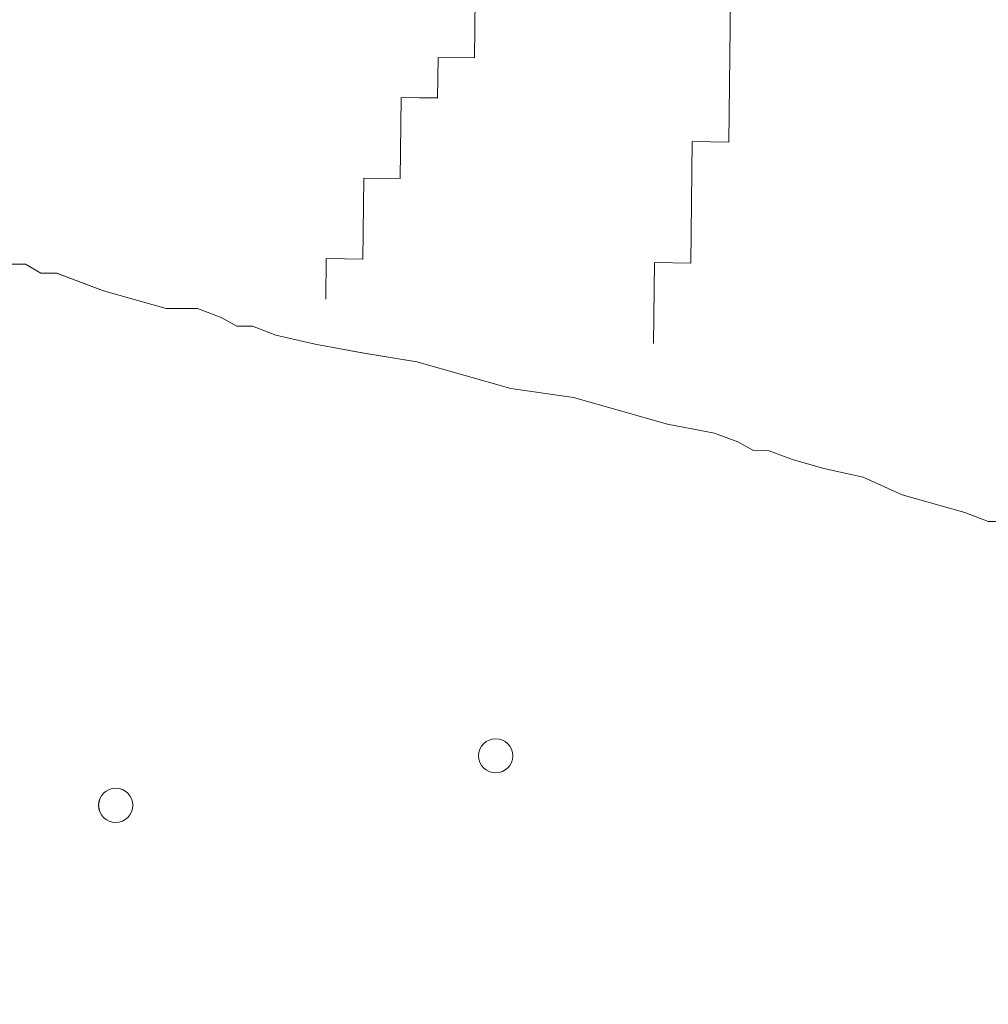
# Model space of a CAD drawing. Units: inches. Extents: x -466983 to 1020, y 324 to 318697.
# Tile 68 of 97: x 643.839 to 647.144, y 939.297 to 942.656. Entities that reach past the tile are written whole.
import ezdxf

# ---------------------------------------------------------------- set-up
doc = ezdxf.new("R2010")
doc.units = ezdxf.units.IN
doc.header["$MEASUREMENT"] = 0
doc.layers.add('A-FLOR-PATT', color=252, linetype='Continuous', lineweight=13)
doc.layers.add('A-FURN', color=8, linetype='Continuous', lineweight=18)

# ---------------------------------------------------------------- blocks, each defined once
blk = doc.blocks.new('L Shaped Sofa')
at = {"ltscale": 2}
for p, q in [((2412.5291, 746.9312), (2412.6267, 746.9307)), ((2412.6267, 746.9307), (2412.7727, 746.8758)), ((2412.7727, 746.8758), (2413.1624, 746.7656)), ((2413.1624, 746.7656), (2413.4057, 746.656)), ((2413.4057, 746.656), (2413.6494, 746.6006)), ((2413.6494, 746.6006), (2413.8442, 746.5455)), ((2413.8442, 746.5455), (2413.9903, 746.4906)), ((2413.9903, 746.4906), (2414.0879, 746.4901)), ((2414.0879, 746.4901), (2414.1851, 746.4354)), ((2414.1851, 746.4354), (2414.3312, 746.3805)), ((2414.3312, 746.3805), (2414.6236, 746.325)), ((2414.6236, 746.325), (2415.2082, 746.1596)), ((2415.2082, 746.1596), (2415.5982, 746.1035)), ((2415.5982, 746.1035), (2416.1827, 745.9381)), ((2416.1827, 745.9381), (2416.524, 745.8823)), ((2416.524, 745.8823), (2416.8164, 745.8267)), ((2414.7046, 745.3203), (2414.7108, 745.8242)), ((2416.8164, 745.8267), (2417.0601, 745.7713)), ((2417.0601, 745.7713), (2417.2061, 745.7164)), ((2417.2061, 745.7164), (2417.3037, 745.716)), ((2417.3037, 745.716), (2417.401, 745.6613)), ((2417.401, 745.6613), (2417.547, 745.6064)), ((2417.547, 745.6064), (2417.7422, 745.6055)), ((2417.7422, 745.6055), (2418.1319, 745.4952)), ((2416.7462, 745.2954), (2416.7493, 745.5473)), ((2418.1319, 745.4952), (2418.424, 745.3854)), ((2418.424, 745.3854), (2418.5216, 745.385)), ((2418.5216, 745.385), (2418.6188, 745.3303)), ((2418.6188, 745.3303), (2418.7164, 745.3298)), ((2414.4686, 744.5674), (2414.4778, 745.3231)), ((2414.4778, 745.3231), (2414.7046, 745.3203)), ((2416.5132, 744.7943), (2416.5193, 745.2982)), ((2416.5193, 745.2982), (2416.7462, 745.2954)), ((2416.2802, 744.2933), (2416.2863, 744.7971)), ((2416.2863, 744.7971), (2416.5132, 744.7943)), ((2414.2017, 741.2953), (2414.2417, 744.5701)), ((2414.2417, 744.5701), (2414.4686, 744.5674)), ((2416.0503, 744.0441), (2416.0534, 744.2961)), ((2416.0534, 744.2961), (2416.2802, 744.2933)), ((2415.8142, 743.2912), (2415.8234, 744.0469)), ((2415.8234, 744.0469), (2416.0503, 744.0441))]:
    blk.add_line(p, q, dxfattribs=at)
for centre, start, end in [((2418.0565, 748.697), 90, 270), ((2418.0565, 748.697), 270, 90), ((2415.692, 748.3889), 90, 270), ((2415.692, 748.3889), 270, 90)]:
    blk.add_arc(centre, 0.1062, start, end, dxfattribs=at)

msp = doc.modelspace()

# ---------------------------------------------------------------- hatches: boundary and pattern name
at = {"layer": 'A-FLOR-PATT', "transparency": 33554572}
h = msp.add_hatch(dxfattribs=at)
h.set_pattern_fill('ANSI37', color=256, scale=30)
h.set_pattern_definition([(45, (-1212.4137, -290.035), (-2.6516504, 2.6516504), []), (135, (-1212.4137, -290.035), (-2.6516504, -2.6516504), [])])
h.paths.add_polyline_path([(901.8057, 1075.9377), (900.6144, 1075.9377), (900.6144, 1065.3856), (899.391, 1065.3856), (898.0911, 1065.3856), (892.8356, 1058.7098, -0.258377), (892.1875, 1058.3509), (879.9848, 1058.3509, -0.20177), (879.4382, 1058.5808), (874.0812, 1065.3856), (872.7813, 1065.3856), (871.5579, 1065.3856), (871.5579, 1075.9377), (813.8057, 1075.9377), (813.8057, 1044.7922), (832.3947, 1044.7922, -0.394795), (848.6602, 1028.5356), (848.6602, 1009.9377), (901.8057, 1009.9377), (901.8057, 1015.9377), (901.3057, 1015.9377), (871.3057, 1015.9377), (871.3057, 1017.2502), (871.3344, 1017.2502, -0.401453), (901.3057, 1045.9377), (901.8057, 1045.9377)])
edge = h.paths.add_edge_path(flags=16)
edge.add_line((847.7731, 1068.9486), (847.7731, 1073.7088))
edge.add_arc((849.2269, 1073.7088), 1.4538, 90, 180, ccw=False)
edge.add_line((849.2269, 1075.1627), (864.4921, 1075.1627))
edge.add_arc((864.4921, 1073.7088), 1.4538, 0, 90, ccw=False)
edge.add_line((865.9459, 1073.7088), (865.9459, 1069.0035))
edge.add_arc((832.6447, 1068.9761), 33.3012, -20.61234, 0.04725, ccw=False)
edge.add_ellipse((856.8595, 1058.48), major_axis=(0, 10.2131), ratio=0.6859192, start_angle=100.00884, end_angle=259.99116, ccw=False)
edge.add_arc((881.0742, 1068.9761), 33.3012, 180.04725, 200.61234, ccw=False)
h.paths.add_polyline_path([(853.1456, 1066.4815), (853.1456, 1066.4534), (853.1463, 1066.4534, 0.433107), (852.9166, 1066.6849), (852.9166, 1066.4534), (853.1456, 1066.4534), (853.1456, 1066.4815), (853.088, 1066.6122, 0.697939), (852.6995, 1066.4534), (852.7003, 1066.4534), (852.7003, 1066.4815), (852.9166, 1067.0012), (852.9166, 1066.6849, -0.396254)], flags=0)
h.paths.add_polyline_path([(861.0187, 1066.4815), (861.0187, 1066.4534), (861.0194, 1066.4534, 0.416404), (860.8024, 1066.6849), (860.8024, 1066.4534), (861.0187, 1066.4534), (861.0187, 1066.4815), (860.9672, 1066.6053, 0.713344), (860.5726, 1066.4534), (860.5734, 1066.4534), (860.5734, 1066.4815), (860.8024, 1067.0012), (860.8024, 1066.6849, -0.379973)], flags=0)
edge = h.paths.add_edge_path(flags=0)
edge.add_spline(control_points=[(861.1298, 1065.7855), (861.4661, 1065.2478), (861.6134, 1065.0161), (861.9833, 1064.3736), (862.1924, 1063.9443), (862.5614, 1063.0391), (862.7212, 1062.5633), (862.9865, 1061.5781), (863.092, 1061.0689), (863.2452, 1060.031), (863.293, 1059.5025), (863.3295, 1058.4409), (863.3181, 1057.9078), (863.2366, 1056.8518), (863.1664, 1056.3289), (862.9695, 1055.308), (862.8427, 1054.8099), (862.5365, 1053.8522), (862.3571, 1053.3927), (861.9514, 1052.5249), (861.7251, 1052.1166), (861.233, 1051.3622), (860.9672, 1051.0162), (860.4048, 1050.3949), (860.1082, 1050.1197), (859.4937, 1049.6461), (859.1758, 1049.4476), (858.5276, 1049.1299), (858.1973, 1049.0107), (857.5315, 1048.8518), (857.1959, 1048.8121), (856.5249, 1048.812), (856.1894, 1048.8515), (855.5236, 1049.0101), (855.1933, 1049.1291), (854.545, 1049.4465), (854.2271, 1049.6449), (853.6124, 1050.1183), (853.3158, 1050.3933), (852.7533, 1051.0143), (852.4874, 1051.3602), (851.9952, 1052.1144), (851.7688, 1052.5225), (851.3629, 1053.3902), (851.1834, 1053.8496), (850.877, 1054.8071), (850.7501, 1055.3051), (850.553, 1056.326), (850.4827, 1056.8488), (850.401, 1057.9048), (850.3895, 1058.4379), (850.4257, 1059.4995), (850.4734, 1060.0281), (850.6265, 1061.066), (850.7318, 1061.5753), (850.9969, 1062.5605), (851.1567, 1063.0365), (851.5254, 1063.9418), (851.7345, 1064.3712), (852.1056, 1065.0164), (852.2544, 1065.2503), (852.6082, 1065.7335)], knot_values=[3.915332, 3.915332, 3.915332, 3.915332, 4.013468, 4.013468, 4.175532, 4.175532, 4.337596, 4.337596, 4.49966, 4.49966, 4.661724, 4.661724, 4.823788, 4.823788, 4.985852, 4.985852, 5.147916, 5.147916, 5.30998, 5.30998, 5.472044, 5.472044, 5.634109, 5.634109, 5.796173, 5.796173, 5.958237, 5.958237, 6.120301, 6.120301, 6.282365, 6.282365, 6.444429, 6.444429, 6.606493, 6.606493, 6.768557, 6.768557, 6.930621, 6.930621, 7.092685, 7.092685, 7.254749, 7.254749, 7.416813, 7.416813, 7.578878, 7.578878, 7.740942, 7.740942, 7.903006, 7.903006, 8.06507, 8.06507, 8.227134, 8.227134, 8.389198, 8.389198, 8.551262, 8.551262, 8.65037, 8.65037, 8.65037, 8.65037], degree=3, periodic=0)
edge.add_line((852.6421, 1065.7855), (861.1298, 1065.7855))
edge = h.paths.add_edge_path(flags=0)
edge.add_ellipse((856.8496, 1057.7432), major_axis=(0, 7.7921), ratio=0.687861, start_angle=0, end_angle=360)
h.paths.add_polyline_path([(848.8634, 1069.3891), (848.8634, 1073.9605, -0.414214), (849.9538, 1075.0508), (863.7652, 1075.0508, -0.414214), (864.8555, 1073.9605), (864.8555, 1069.3891, -0.388936), (864.5237, 1069.027, -0.043561), (849.1953, 1069.027, -0.388936)], flags=0)
h.paths.add_polyline_path([(853.1006, 1068.1122, -1), (852.6775, 1068.1122, -1)], flags=0)
edge = h.paths.add_edge_path(flags=0)
edge.add_ellipse((856.8595, 1057.3378), major_axis=(0, 2.207), ratio=0.657164, start_angle=0, end_angle=360)
h.paths.add_polyline_path([(861.0415, 1068.1122, -1), (860.6184, 1068.1122, -1)], flags=0)
edge = h.paths.add_edge_path()
edge.add_line((573.9537, 1057.3412), (573.9537, 1075.9377))
edge.add_line((573.9537, 1075.9377), (558.7308, 1075.9377))
edge.add_line((558.7308, 1075.9377), (558.7308, 1065.3856))
edge.add_line((558.7308, 1065.3856), (557.5074, 1065.3856))
edge.add_line((557.5074, 1065.3856), (556.2075, 1065.3856))
edge.add_line((556.2075, 1065.3856), (550.952, 1058.7098))
edge.add_arc((550.3039, 1059.1155), 0.7646, 270, 327.9483, ccw=False)
edge.add_line((550.3039, 1058.3509), (538.1012, 1058.3509))
edge.add_arc((538.1012, 1059.1155), 0.7646, 224.3704, 270, ccw=False)
edge.add_line((537.5546, 1058.5808), (532.1976, 1065.3856))
edge.add_line((532.1976, 1065.3856), (530.8977, 1065.3856))
edge.add_line((530.8977, 1065.3856), (529.6743, 1065.3856))
edge.add_line((529.6743, 1065.3856), (529.6743, 1075.9377))
edge.add_line((529.6743, 1075.9377), (520.8057, 1075.9377))
edge.add_line((520.8057, 1075.9377), (520.8057, 1045.9377))
edge.add_line((520.8057, 1045.9377), (521.3057, 1045.9377))
edge.add_arc((521.3057, 1015.9377), 30, 2.50749, 90, ccw=False)
edge.add_line((551.277, 1017.2502), (551.3057, 1017.2502))
edge.add_line((551.3057, 1017.2502), (551.3057, 1015.9377))
edge.add_line((551.3057, 1015.9377), (520.8057, 1015.9377))
edge.add_line((520.8057, 1015.9377), (520.8057, 1009.9377))
edge.add_line((520.8057, 1009.9377), (559.1913, 1010.4022))
edge.add_arc((559.1913, 1011.856), 1.4538, 180, 270, ccw=False)
edge.add_line((557.7375, 1011.856), (557.7375, 1016.5613))
edge.add_arc((591.0386, 1016.5888), 33.3012, 159.38766, 180.04725, ccw=False)
edge.add_ellipse((566.8239, 1027.0848), major_axis=(0, 10.2131), ratio=0.6859192, start_angle=280.00884, end_angle=439.99116, ccw=False)
edge.add_arc((542.6091, 1016.5888), 33.3012, 0.04725, 20.61234, ccw=False)
edge.add_line((575.9103, 1016.6162), (575.9103, 1011.856))
edge.add_arc((574.4565, 1011.856), 1.4538, -90, 0, ccw=False)
edge.add_line((574.4565, 1010.4022), (608.8057, 1009.9377))
edge.add_line((608.8057, 1009.9377), (608.8057, 1041.0857))
edge.add_line((608.8057, 1041.0857), (590.2179, 1041.0857))
edge.add_arc((590.775, 1057.9074), 16.8309, 181.92775, 268.10321, ccw=False)
edge = h.paths.add_edge_path()
edge.add_ellipse((494.2443, 583.6204), major_axis=(0, 10.2131), ratio=0.6859192, start_angle=280.00884, end_angle=439.99116, ccw=False)
edge.add_arc((470.0296, 573.1243), 33.3012, 0.04725, 20.61234, ccw=False)
edge.add_line((503.3307, 573.1518), (503.3307, 568.3916))
edge.add_arc((501.8769, 568.3916), 1.4538, -90, 0, ccw=False)
edge.add_line((501.8769, 566.9377), (539.8057, 566.9377))
edge.add_line((539.8057, 566.9377), (539.8057, 572.9377))
edge.add_line((539.8057, 572.9377), (539.3057, 572.9377))
edge.add_line((539.3057, 572.9377), (509.3057, 572.9377))
edge.add_line((509.3057, 572.9377), (509.3057, 574.2502))
edge.add_line((509.3057, 574.2502), (509.3344, 574.2502))
edge.add_arc((539.3057, 572.9377), 30, 90, 177.49251, ccw=False)
edge.add_line((539.3057, 602.9377), (539.8057, 602.9377))
edge.add_line((539.8057, 602.9377), (539.8057, 626.9377))
edge.add_line((539.8057, 626.9377), (531.7718, 626.9377))
edge.add_line((531.7718, 626.9377), (531.7718, 616.3856))
edge.add_line((531.7718, 616.3856), (530.5484, 616.3856))
edge.add_line((530.5484, 616.3856), (529.2485, 616.3856))
edge.add_line((529.2485, 616.3856), (523.7105, 609.3509))
edge.add_line((523.7105, 609.3509), (510.7766, 609.3509))
edge.add_line((510.7766, 609.3509), (505.2386, 616.3856))
edge.add_line((505.2386, 616.3856), (503.9387, 616.3856))
edge.add_line((503.9387, 616.3856), (502.7153, 616.3856))
edge.add_line((502.7153, 616.3856), (502.7153, 626.9377))
edge.add_line((502.7153, 626.9377), (481.6983, 626.9377))
edge.add_line((481.6983, 626.9377), (481.6983, 610.995))
edge.add_arc((467.2703, 611.4728), 14.4359, 271.92775, 358.10321, ccw=False)
edge.add_line((467.7559, 597.0451), (451.8057, 597.0451))
edge.add_line((451.8057, 597.0451), (451.8057, 584.4035))
edge.add_line((451.8057, 584.4035), (451.8057, 566.9377))
edge.add_line((451.8057, 566.9377), (486.6117, 566.9377))
edge.add_arc((486.6117, 568.3916), 1.4538, 180, 270, ccw=False)
edge.add_line((485.1579, 568.3916), (485.1579, 573.0969))
edge.add_arc((518.4591, 573.1243), 33.3012, 159.38766, 180.04725, ccw=False)
h.paths.add_polyline_path([(836.2609, 1020.7328), (879.8898, 1020.7328), (879.8898, 1039.3902), (836.2609, 1039.3902)], flags=25)
h.paths.add_polyline_path([(549.9851, 1036.7492), (593.614, 1036.7492), (593.614, 1055.4065), (549.9851, 1055.4065)], flags=24)
h.paths.add_polyline_path([(475.123, 595.5959), (518.752, 595.5959), (518.752, 614.2532), (475.123, 614.2532)], flags=24)
h = msp.add_hatch(dxfattribs=at)
h.set_pattern_fill('ANSI37', color=256, scale=20)
h.set_pattern_definition([(45, (-1212.4137, -290.035), (-1.767767, 1.767767), []), (135, (-1212.4137, -290.035), (-1.767767, -1.767767), [])])
h.paths.add_polyline_path([(809.8057, 870.9377), (809.8057, 888.1519), (806.9985, 888.1519), (802.6624, 888.1519), (789.3832, 888.1519), (786.2846, 888.1519, -0.414214), (785.4991, 888.9374), (785.4991, 900.1959), (785.4991, 908.4696, -0.414214), (786.8082, 909.7787, -0.414214), (785.4991, 911.0878), (785.4991, 929.1015, -0.414214), (786.8082, 930.4106, -0.414214), (785.4991, 931.7197), (785.4991, 931.9039, -0.414214), (784.19, 930.5948), (766.7223, 930.5948, -0.412359), (765.4132, 931.8956, -0.413741), (764.1145, 930.5782), (744.5781, 930.422, -0.416556), (743.7864, 931.2075), (743.7864, 933.5153), (742.2154, 933.5153), (742.2154, 952.024, -0.001344), (743.7864, 952.1998), (743.7864, 953.9377), (678.5915, 953.9377), (678.5915, 951.1305), (678.5915, 946.7945), (678.5915, 933.5153), (678.5915, 930.4166, -0.414214), (677.806, 929.6312), (666.5475, 929.6312), (658.2738, 929.6312, -0.414214), (656.9647, 930.9403, -0.414214), (655.6556, 929.6312), (637.6419, 929.6312, -0.414214), (636.3328, 930.9403, -0.414214), (635.0237, 929.6312), (634.8395, 929.6312, -0.414214), (636.1486, 928.322), (636.1486, 910.8544, -0.412359), (634.8478, 909.5452, -0.413741), (636.1653, 908.2466), (636.3214, 888.7102, -0.416556), (635.5359, 887.9184), (633.2281, 887.9184), (633.2281, 886.3475), (614.7194, 886.3475, -0.001344), (614.5436, 887.9184), (612.8057, 887.9184), (612.8057, 834.9377), (612.8057, 752.9377), (612.8057, 748.9377), (612.8057, 697.9377), (654.8057, 697.9377), (654.8057, 701.9377), (715.8057, 701.9377), (715.8057, 737.4353), (774.2918, 737.4353), (774.2918, 795.9377), (809.8057, 795.9377)])
h.paths.add_polyline_path([(679.2761, 849.5757, 0.102523), (682.1475, 849.2608, -0.080461), (694.5428, 849.7725, -0.283899), (694.4822, 849.0082, 0.136605), (694.4068, 848.8103, -0.030441), (694.5428, 846.8929), (694.5428, 842.6198), (694.5428, 838.3466, -0.028219), (694.4246, 836.5684), (694.425, 836.5684, 0.196187), (694.4456, 836.2708, -0.302897), (694.5428, 835.467, -0.080461), (682.1475, 835.9787, 0.102523), (679.2761, 835.6638, -0.58611), (678.6457, 836.0169), (678.6457, 849.2227, -0.58611)], flags=16)
h.paths.add_polyline_path([(679.5173, 848.6515, 0.699597), (679.476, 848.6342, 1.20716), (679.1935, 848.7422, 0.010621)], flags=0)
h.paths.add_polyline_path([(679.4923, 836.5608, -0.013798), (679.9178, 836.6594, -0.071703), (682.8533, 837.1434, -0.165743), (682.1665, 839.1006), (682.1665, 842.6094), (682.1665, 846.0603, -0.240616), (683.4733, 848.6767, -0.068263), (693.9295, 849.0082), (693.7875, 848.7083), (693.7875, 849.0228, 0.067332), (683.4733, 848.6767, 0.240616), (682.1665, 846.0603), (682.1665, 842.6094), (682.1665, 839.1006, 0.23459), (683.461, 836.5513, 0.068093), (693.7875, 836.1955), (693.7875, 836.5104), (693.9296, 836.2102, -0.077215), (682.2421, 836.7815, 0.086627), (679.5283, 836.5701, -0.628402), (679.5029, 836.5735), (679.5029, 836.6071, 0.910458)], flags=0)
h.paths.add_polyline_path([(679.476, 848.6364), (679.2069, 848.647), (679.2069, 836.5718, 0.913566), (679.3645, 836.5861), (679.476, 836.5824)], flags=0)
h.paths.add_polyline_path([(679.2761, 829.8604, 0.102523), (682.1475, 829.5455, -0.080461), (694.5428, 830.0572, -0.283899), (694.4822, 829.2929, 0.136605), (694.4068, 829.095, -0.030441), (694.5428, 827.1776), (694.5428, 822.9045), (694.5428, 818.6314, -0.028219), (694.4246, 816.8531), (694.425, 816.8532, 0.196187), (694.4456, 816.5555, -0.302897), (694.5428, 815.7517, -0.080461), (682.1475, 816.2635, 0.102523), (679.2761, 815.9485, -0.58611), (678.6457, 816.3016), (678.6457, 829.5074, -0.58611)], flags=16)
h.paths.add_polyline_path([(679.5173, 828.9362, 0.699597), (679.476, 828.9189, 1.20716), (679.1935, 829.0269, 0.010621)], flags=0)
h.paths.add_polyline_path([(679.4923, 816.8456, -0.013798), (679.9178, 816.9441, -0.071703), (682.8533, 817.4281, -0.165743), (682.1665, 819.3853), (682.1665, 822.8941), (682.1665, 826.345, -0.240616), (683.4733, 828.9614, -0.068263), (693.9295, 829.2929), (693.7875, 828.9931), (693.7875, 829.3076, 0.067332), (683.4733, 828.9614, 0.240616), (682.1665, 826.345), (682.1665, 822.8941), (682.1665, 819.3853, 0.23459), (683.461, 816.836, 0.068093), (693.7875, 816.4802), (693.7875, 816.7952), (693.9296, 816.4949, -0.077215), (682.2421, 817.0662, 0.086627), (679.5283, 816.8549, -0.628402), (679.5029, 816.8582), (679.5029, 816.8918, 0.910458)], flags=0)
h.paths.add_polyline_path([(679.476, 828.9211), (679.2069, 828.9317), (679.2069, 816.8565, 0.913566), (679.3645, 816.8708), (679.476, 816.8671)], flags=0)
h.paths.add_polyline_path([(679.2761, 810.1451, 0.102523), (682.1475, 809.8302, -0.080461), (694.5428, 810.342, -0.3023), (694.4466, 809.5394, 0.10023), (694.4058, 809.3878, -0.03057), (694.5428, 807.4623), (694.5428, 803.1892), (694.5428, 798.9161, -0.03057), (694.4058, 796.9906, 0.10023), (694.4466, 796.839, -0.3023), (694.5428, 796.0365, -0.080461), (682.1475, 796.5482, 0.102523), (679.2761, 796.2333, -0.58611), (678.6457, 796.5863), (678.6457, 809.7921, -0.58611)], flags=16)
h.paths.add_polyline_path([(679.5173, 809.2417, 0.699597), (679.476, 809.2244, 1.20716), (679.1935, 809.3324, 0.010621)], flags=0)
h.paths.add_polyline_path([(679.4923, 797.151, -0.013798), (679.9178, 797.2496, -0.071703), (682.8533, 797.7336, -0.165743), (682.1665, 799.6908), (682.1665, 803.1996), (682.1665, 806.6505, -0.239349), (683.461, 809.2577, -0.072465), (694.4468, 809.5405, 0.197932), (694.425, 809.2405), (693.7875, 809.2985), (693.7875, 809.6135, 0.068093), (683.461, 809.2577, 0.239349), (682.1665, 806.6505), (682.1665, 803.1996), (682.1665, 799.6908, 0.235854), (683.4733, 797.1323, 0.067332), (693.7875, 796.7861), (693.7875, 797.1006), (694.425, 797.1586, 0.197932), (694.4468, 796.8586, -0.080419), (682.1557, 797.3795, 0.083867), (679.5283, 797.1603, -0.628402), (679.5029, 797.1637), (679.5029, 797.1973, 0.910458)], flags=0)
h.paths.add_polyline_path([(679.2069, 809.2372), (679.2069, 797.162, 0.913566), (679.3645, 797.1763), (679.476, 797.1726), (679.476, 809.2266)], flags=0)
h.paths.add_polyline_path([(695.3643, 853.2989), (728.2231, 853.2989), (728.2231, 771.1519), (695.3643, 771.1519)], flags=16)
h.paths.add_polyline_path([(696.0215, 852.6417), (727.5659, 852.6417), (727.5659, 771.809), (696.0215, 771.809)], flags=0)
h.paths.add_polyline_path([(679.2761, 788.7869, 0.102523), (682.1475, 788.472, -0.080461), (694.5428, 788.9837, -0.3023), (694.4466, 788.1812, 0.10023), (694.4058, 788.0296, -0.03057), (694.5428, 786.1041), (694.5428, 781.831), (694.5428, 777.5578, -0.03057), (694.4058, 775.6323, 0.10023), (694.4466, 775.4808, -0.3023), (694.5428, 774.6782, -0.080461), (682.1475, 775.19, 0.102523), (679.2761, 774.875, -0.58611), (678.6457, 775.2281), (678.6457, 788.4339, -0.58611)], flags=16)
h.paths.add_polyline_path([(679.5173, 787.8834, 0.699597), (679.476, 787.8662, 1.20716), (679.1935, 787.9742, 0.010621)], flags=0)
h.paths.add_polyline_path([(679.4923, 775.7928, -0.013798), (679.9178, 775.8914, -0.071703), (682.8533, 776.3753, -0.165743), (682.1665, 778.3325), (682.1665, 781.8414), (682.1665, 785.2922, -0.239349), (683.461, 787.8995, -0.072465), (694.4468, 788.1823, 0.197932), (694.425, 787.8823), (693.7875, 787.9403), (693.7875, 788.2553, 0.068093), (683.461, 787.8995, 0.239349), (682.1665, 785.2922), (682.1665, 781.8414), (682.1665, 778.3325, 0.235854), (683.4733, 775.7741, 0.067332), (693.7875, 775.4279), (693.7875, 775.7424), (694.425, 775.8004, 0.197932), (694.4468, 775.5004, -0.080419), (682.1557, 776.0212, 0.083867), (679.5283, 775.8021, -0.628402), (679.5029, 775.8054), (679.5029, 775.8391, 0.910458)], flags=0)
h.paths.add_polyline_path([(679.2069, 787.8789), (679.2069, 775.8038, 0.913566), (679.3645, 775.818), (679.476, 775.8144), (679.476, 787.8684)], flags=0)
h.paths.add_polyline_path([(704.641, 854.1204, -0.080461), (705.1527, 866.5157, 0.102523), (704.8378, 869.3871, -0.58611), (705.1908, 870.0174), (718.3966, 870.0174, -0.58611), (718.7496, 869.3871, 0.102523), (718.4347, 866.5157, -0.080461), (718.9465, 854.1204, -0.3023), (718.1439, 854.2166, 0.10023), (717.9924, 854.2574, -0.03057), (716.0668, 854.1204), (711.7937, 854.1204), (707.5206, 854.1204, -0.03057), (705.5951, 854.2574, 0.10023), (705.4435, 854.2166, -0.3023)], flags=16)
h.paths.add_polyline_path([(717.8462, 869.1459, 0.699597), (717.8289, 869.1872, 1.20716), (717.9369, 869.4697, 0.010621)], flags=0)
h.paths.add_polyline_path([(705.4631, 854.2164, -0.080419), (705.984, 866.5074, 0.083867), (705.7648, 869.1349, -0.628402), (705.7682, 869.1603), (705.8018, 869.1603, 0.910458), (705.7555, 869.1709, -0.013798), (705.8541, 868.7454, -0.071703), (706.3381, 865.8099, -0.165743), (708.2953, 866.4967), (711.8041, 866.4967), (715.255, 866.4967, -0.239349), (717.8622, 865.2022, -0.072465), (718.145, 854.2164, 0.197932), (717.845, 854.2382), (717.903, 854.8757), (718.218, 854.8757, 0.068093), (717.8622, 865.2022, 0.239349), (715.255, 866.4967), (711.8041, 866.4967), (708.2953, 866.4967, 0.235854), (705.7368, 865.1898, 0.067332), (705.3906, 854.8757), (705.7051, 854.8757), (705.7631, 854.2382, 0.197932)], flags=16)
h.paths.add_polyline_path([(705.7665, 869.4563, 0.913566), (705.7808, 869.2987), (705.7771, 869.1872), (717.8311, 869.1872), (717.8417, 869.4563)], flags=0)
h.paths.add_polyline_path([(729.0446, 842.6198), (729.0446, 846.8929, -0.03057), (729.1817, 848.8184, 0.10023), (729.1408, 848.9699, -0.3023), (729.0446, 849.7725, -0.080461), (741.4399, 849.2608, 0.102523), (744.3113, 849.5757, -0.58611), (744.9417, 849.2227), (744.9417, 836.0169, -0.58611), (744.3113, 835.6638, 0.102523), (741.4399, 835.9787, -0.080461), (729.0446, 835.467, -0.3023), (729.1408, 836.2696, 0.10023), (729.1817, 836.4211, -0.03057), (729.0446, 838.3466)], flags=16)
h.paths.add_polyline_path([(744.1115, 836.5846, 1.20716), (744.3939, 836.4766, 0.010621), (744.0701, 836.5673, 0.699597)], flags=0)
h.paths.add_polyline_path([(729.1407, 836.2684, 0.197932), (729.1624, 836.5684), (729.7999, 836.5104), (729.7999, 836.1955, 0.068093), (740.1264, 836.5513, 0.239349), (741.4209, 839.1585), (741.4209, 842.6094), (741.4209, 846.1182, 0.235854), (740.1141, 848.6767, 0.067332), (729.7999, 849.0228), (729.7999, 848.7083), (729.1624, 848.6503, 0.197932), (729.1407, 848.9504, -0.080419), (741.4317, 848.4295, 0.083867), (744.0591, 848.6486, -0.628402), (744.0845, 848.6453), (744.0845, 848.6117, 0.910458), (744.0951, 848.6579, -0.013798), (743.6696, 848.5594, -0.071703), (740.7341, 848.0754, -0.165743), (741.4209, 846.1182), (741.4209, 842.6094), (741.4209, 839.1585, -0.239349), (740.1264, 836.5513, -0.072465)], flags=0)
h.paths.add_polyline_path([(729.0446, 830.0572, -0.080461), (741.4399, 829.5455, 0.102523), (744.3113, 829.8604, -0.58611), (744.9417, 829.5074), (744.9417, 816.3016, -0.58611), (744.3113, 815.9485, 0.102523), (741.4399, 816.2635, -0.080461), (729.0446, 815.7517, -0.3023), (729.1408, 816.5543, 0.10023), (729.1817, 816.7058, -0.03057), (729.0446, 818.6314), (729.0446, 822.9045), (729.0446, 827.1776, -0.03057), (729.1817, 829.1031, 0.10023), (729.1408, 829.2547, -0.3023)], flags=16)
h.paths.add_polyline_path([(744.1115, 816.8693, 1.20716), (744.3939, 816.7613, 0.010621), (744.0701, 816.852, 0.699597)], flags=0)
h.paths.add_polyline_path([(729.1407, 829.2351, -0.080419), (741.4317, 828.7142, 0.083867), (744.0591, 828.9334, -0.628402), (744.0845, 828.93), (744.0845, 828.8964, 0.910458), (744.0951, 828.9427, -0.013798), (743.6696, 828.8441, -0.071703), (740.7341, 828.3601, -0.165743), (741.4209, 826.4029), (741.4209, 822.8941), (741.4209, 819.4432, -0.239349), (740.1264, 816.836, -0.072465), (729.1407, 816.5531, 0.197932), (729.1624, 816.8532), (729.7999, 816.7952), (729.7999, 816.4802, 0.068093), (740.1264, 816.836, 0.239349), (741.4209, 819.4432), (741.4209, 822.8941), (741.4209, 826.4029, 0.235854), (740.1141, 828.9614, 0.067332), (729.7999, 829.3076), (729.7999, 828.9931), (729.1624, 828.9351, 0.197932)], flags=16)
h.paths.add_polyline_path([(729.0446, 810.342, -0.080461), (741.4399, 809.8302, 0.102523), (744.3113, 810.1451, -0.58611), (744.9417, 809.7921), (744.9417, 796.5863, -0.58611), (744.3113, 796.2333, 0.102523), (741.4399, 796.5482, -0.080461), (729.0446, 796.0365, -0.283899), (729.1052, 796.8007, 0.136605), (729.1806, 796.9987, -0.030441), (729.0446, 798.9161), (729.0446, 803.1892), (729.0446, 807.4623, -0.028219), (729.1628, 809.2406), (729.1624, 809.2405, 0.196187), (729.1418, 809.5382, -0.302897)], flags=16)
h.paths.add_polyline_path([(744.1115, 797.1748, 1.20716), (744.3939, 797.0668, 0.010621), (744.0701, 797.1575, 0.699597)], flags=0)
h.paths.add_polyline_path([(741.3453, 809.0275, 0.086627), (744.0591, 809.2388, -0.628402), (744.0845, 809.2355), (744.0845, 809.2019, 0.910458), (744.0951, 809.2481, -0.013798), (743.6696, 809.1496, -0.071703), (740.7341, 808.6656, -0.165743), (741.4209, 806.7084), (741.4209, 803.1996), (741.4209, 799.7487, -0.240616), (740.1141, 797.1323, -0.068263), (729.658, 796.8008), (729.7999, 797.1006), (729.7999, 796.7861, 0.067332), (740.1141, 797.1323, 0.240616), (741.4209, 799.7487), (741.4209, 803.1996), (741.4209, 806.7084, 0.23459), (740.1264, 809.2577, 0.068093), (729.7999, 809.6135), (729.7999, 809.2985), (729.6578, 809.5988, -0.077215)], flags=0)
h.paths.add_polyline_path([(704.641, 770.3304, -0.283899), (705.4053, 770.2697, 0.136605), (705.6032, 770.1944, -0.030441), (707.5206, 770.3304), (711.7937, 770.3304), (716.0668, 770.3304, -0.028219), (717.8451, 770.2122), (717.845, 770.2126, 0.196187), (718.1427, 770.2331, -0.302897), (718.9465, 770.3304, -0.080461), (718.4347, 757.9351, 0.102523), (718.7496, 755.0637, -0.58611), (718.3966, 754.4333), (705.1908, 754.4333, -0.58611), (704.8378, 755.0637, 0.102523), (705.1527, 757.9351, -0.080461)], flags=16)
h.paths.add_polyline_path([(705.762, 755.3048, 0.699597), (705.7793, 755.2635, 1.20716), (705.6713, 754.9811, 0.010621)], flags=0)
h.paths.add_polyline_path([(705.4053, 769.717), (705.7051, 769.5751), (705.3906, 769.5751, 0.067332), (705.7368, 759.2609, 0.240616), (708.3532, 757.954), (711.8041, 757.954), (715.3129, 757.954, 0.23459), (717.8622, 759.2485, 0.068093), (718.218, 769.5751), (717.903, 769.5751), (718.2033, 769.7172, -0.077215), (717.632, 758.0297, 0.086627), (717.8433, 755.3159, -0.628402), (717.84, 755.2904), (717.8064, 755.2904, 0.910458), (717.8526, 755.2799, -0.013798), (717.7541, 755.7053, -0.071703), (717.2701, 758.6409, -0.165743), (715.3129, 757.954), (711.8041, 757.954), (708.3532, 757.954, -0.240616), (705.7368, 759.2609, -0.068263)], flags=0)
h.paths.add_polyline_path([(729.0446, 788.9837, -0.080461), (741.4399, 788.472, 0.102523), (744.3113, 788.7869, -0.58611), (744.9417, 788.4339), (744.9417, 775.2281, -0.58611), (744.3113, 774.875, 0.102523), (741.4399, 775.19, -0.080461), (729.0446, 774.6782, -0.283899), (729.1052, 775.4425, 0.136605), (729.1806, 775.6405, -0.030441), (729.0446, 777.5578), (729.0446, 781.831), (729.0446, 786.1041, -0.028219), (729.1628, 787.8823), (729.1624, 787.8823, 0.196187), (729.1418, 788.1799, -0.302897)], flags=16)
h.paths.add_polyline_path([(744.1115, 775.8165, 1.20716), (744.3939, 775.7086, 0.010621), (744.0701, 775.7993, 0.699597)], flags=0)
h.paths.add_polyline_path([(741.3453, 787.6692, 0.086627), (744.0591, 787.8806, -0.628402), (744.0845, 787.8773), (744.0845, 787.8437, 0.910458), (744.0951, 787.8899, -0.013798), (743.6696, 787.7913, -0.071703), (740.7341, 787.3074, -0.165743), (741.4209, 785.3502), (741.4209, 781.8414), (741.4209, 778.3905, -0.240616), (740.1141, 775.7741, -0.068263), (729.658, 775.4425), (729.7999, 775.7424), (729.7999, 775.4279, 0.067332), (740.1141, 775.7741, 0.240616), (741.4209, 778.3905), (741.4209, 781.8414), (741.4209, 785.3502, 0.23459), (740.1264, 787.8995, 0.068093), (729.7999, 788.2553), (729.7999, 787.9403), (729.6578, 788.2405, -0.077215)], flags=0)
h.paths.add_polyline_path([(744.1115, 848.6364), (744.1115, 836.5824), (744.3805, 836.5718), (744.3805, 848.647, 0.913566), (744.2229, 848.6327)], flags=0)
h.paths.add_polyline_path([(744.2229, 828.9174), (744.1115, 828.9211), (744.1115, 816.8671), (744.3805, 816.8565), (744.3805, 828.9317, 0.913566)], flags=0)
h.paths.add_polyline_path([(717.8311, 755.2635), (705.7771, 755.2635), (705.7665, 754.9945), (717.8417, 754.9945, 0.913566), (717.8274, 755.1521)], flags=0)
h.paths.add_polyline_path([(744.2229, 809.2229), (744.1115, 809.2266), (744.1115, 797.1726), (744.3805, 797.162), (744.3805, 809.2372, 0.913566)], flags=0)
h.paths.add_polyline_path([(744.1115, 787.8684), (744.1115, 775.8144), (744.3805, 775.8038), (744.3805, 787.8789, 0.913566), (744.2229, 787.8647)], flags=0)
h.paths.add_polyline_path([(678.8774, 877.1228), (737.6127, 877.1228), (737.6127, 899.5116), (678.8774, 899.5116)], flags=24)

# ---------------------------------------------------------------- linework, layer by layer
at = {"layer": 'A-FURN', "ltscale": 2}
for p, q in [((646.2803, 944.0337), (646.2584, 942.2384)), ((646.2803, 944.0337), (646.2584, 942.2384)), ((646.2803, 944.0337), (646.2584, 942.2384)), ((646.2803, 944.0337), (646.2584, 942.2384)), ((646.2803, 944.0337), (646.2584, 942.2384)), ((646.2803, 944.0337), (646.2584, 942.2384)), ((645.3963, 942.9396), (645.3913, 942.5253)), ((645.3963, 942.9396), (645.3913, 942.5253)), ((645.3963, 942.9396), (645.3913, 942.5253)), ((645.3963, 942.9396), (645.3913, 942.5253)), ((645.3963, 942.9396), (645.3913, 942.5253)), ((645.3963, 942.9396), (645.3913, 942.5253)), ((645.2669, 942.5268), (645.2652, 942.3887)), ((645.2669, 942.5268), (645.2652, 942.3887)), ((645.2669, 942.5268), (645.2652, 942.3887)), ((645.2669, 942.5268), (645.2652, 942.3887)), ((645.2669, 942.5268), (645.2652, 942.3887)), ((645.2669, 942.5268), (645.2652, 942.3887)), ((645.3913, 942.5253), (645.2669, 942.5268)), ((645.3913, 942.5253), (645.2669, 942.5268)), ((645.3913, 942.5253), (645.2669, 942.5268)), ((645.3913, 942.5253), (645.2669, 942.5268)), ((645.3913, 942.5253), (645.2669, 942.5268)), ((645.3913, 942.5253), (645.2669, 942.5268)), ((645.1409, 942.3902), (645.1375, 942.114)), ((645.1409, 942.3902), (645.1375, 942.114)), ((645.1409, 942.3902), (645.1375, 942.114)), ((645.1409, 942.3902), (645.1375, 942.114)), ((645.1409, 942.3902), (645.1375, 942.114)), ((645.1409, 942.3902), (645.1375, 942.114)), ((645.2652, 942.3887), (645.1409, 942.3902)), ((645.2652, 942.3887), (645.1409, 942.3902)), ((645.2652, 942.3887), (645.1409, 942.3902)), ((645.2652, 942.3887), (645.1409, 942.3902)), ((645.2652, 942.3887), (645.1409, 942.3902)), ((645.2652, 942.3887), (645.1409, 942.3902)), ((646.134, 942.2399), (646.1289, 941.8256)), ((646.134, 942.2399), (646.1289, 941.8256)), ((646.134, 942.2399), (646.1289, 941.8256)), ((646.134, 942.2399), (646.1289, 941.8256)), ((646.134, 942.2399), (646.1289, 941.8256)), ((646.134, 942.2399), (646.1289, 941.8256)), ((646.2584, 942.2384), (646.134, 942.2399)), ((646.2584, 942.2384), (646.134, 942.2399)), ((646.2584, 942.2384), (646.134, 942.2399)), ((646.2584, 942.2384), (646.134, 942.2399)), ((646.2584, 942.2384), (646.134, 942.2399)), ((646.2584, 942.2384), (646.134, 942.2399)), ((645.0131, 942.1155), (645.0097, 941.8393)), ((645.0131, 942.1155), (645.0097, 941.8393)), ((645.0131, 942.1155), (645.0097, 941.8393)), ((645.0131, 942.1155), (645.0097, 941.8393)), ((645.0131, 942.1155), (645.0097, 941.8393)), ((645.0131, 942.1155), (645.0097, 941.8393)), ((645.1375, 942.114), (645.0131, 942.1155)), ((645.1375, 942.114), (645.0131, 942.1155)), ((645.1375, 942.114), (645.0131, 942.1155)), ((645.1375, 942.114), (645.0131, 942.1155)), ((645.1375, 942.114), (645.0131, 942.1155)), ((645.1375, 942.114), (645.0131, 942.1155)), ((644.8854, 941.8408), (644.8837, 941.7027)), ((644.8854, 941.8408), (644.8837, 941.7027)), ((644.8854, 941.8408), (644.8837, 941.7027)), ((644.8854, 941.8408), (644.8837, 941.7027)), ((644.8854, 941.8408), (644.8837, 941.7027)), ((644.8854, 941.8408), (644.8837, 941.7027)), ((645.0097, 941.8393), (644.8854, 941.8408)), ((645.0097, 941.8393), (644.8854, 941.8408)), ((645.0097, 941.8393), (644.8854, 941.8408)), ((645.0097, 941.8393), (644.8854, 941.8408)), ((645.0097, 941.8393), (644.8854, 941.8408)), ((645.0097, 941.8393), (644.8854, 941.8408)), ((643.8588, 941.8217), (643.8053, 941.8219)), ((643.8588, 941.8217), (643.8053, 941.8219)), ((643.8588, 941.8217), (643.8053, 941.8219)), ((643.8588, 941.8217), (643.8053, 941.8219)), ((643.8588, 941.8217), (643.8053, 941.8219)), ((643.8588, 941.8217), (643.8053, 941.8219)), ((643.9121, 941.7917), (643.8588, 941.8217)), ((643.9121, 941.7917), (643.8588, 941.8217)), ((643.9121, 941.7917), (643.8588, 941.8217)), ((643.9121, 941.7917), (643.8588, 941.8217)), ((643.9121, 941.7917), (643.8588, 941.8217)), ((643.9121, 941.7917), (643.8588, 941.8217)), ((646.0046, 941.8271), (646.0012, 941.5509)), ((646.0046, 941.8271), (646.0012, 941.5509)), ((646.0046, 941.8271), (646.0012, 941.5509)), ((646.0046, 941.8271), (646.0012, 941.5509)), ((646.0046, 941.8271), (646.0012, 941.5509)), ((646.0046, 941.8271), (646.0012, 941.5509)), ((646.1289, 941.8256), (646.0046, 941.8271)), ((646.1289, 941.8256), (646.0046, 941.8271)), ((646.1289, 941.8256), (646.0046, 941.8271)), ((646.1289, 941.8256), (646.0046, 941.8271)), ((646.1289, 941.8256), (646.0046, 941.8271)), ((646.1289, 941.8256), (646.0046, 941.8271)), ((643.9656, 941.7915), (643.9121, 941.7917)), ((643.9656, 941.7915), (643.9121, 941.7917)), ((643.9656, 941.7915), (643.9121, 941.7917)), ((643.9656, 941.7915), (643.9121, 941.7917)), ((643.9656, 941.7915), (643.9121, 941.7917)), ((643.9656, 941.7915), (643.9121, 941.7917)), ((644.1257, 941.7313), (643.9656, 941.7915)), ((644.1257, 941.7313), (643.9656, 941.7915)), ((644.1257, 941.7313), (643.9656, 941.7915)), ((644.1257, 941.7313), (643.9656, 941.7915)), ((644.1257, 941.7313), (643.9656, 941.7915)), ((644.1257, 941.7313), (643.9656, 941.7915)), ((644.3394, 941.6708), (644.1257, 941.7313)), ((644.3394, 941.6708), (644.1257, 941.7313)), ((644.3394, 941.6708), (644.1257, 941.7313)), ((644.3394, 941.6708), (644.1257, 941.7313)), ((644.3394, 941.6708), (644.1257, 941.7313)), ((644.3394, 941.6708), (644.1257, 941.7313)), ((644.4464, 941.6703), (644.3394, 941.6708)), ((644.4464, 941.6703), (644.3394, 941.6708)), ((644.4464, 941.6703), (644.3394, 941.6708)), ((644.4464, 941.6703), (644.3394, 941.6708)), ((644.4464, 941.6703), (644.3394, 941.6708)), ((644.4464, 941.6703), (644.3394, 941.6708)), ((644.5264, 941.6402), (644.4464, 941.6703)), ((644.5264, 941.6402), (644.4464, 941.6703)), ((644.5264, 941.6402), (644.4464, 941.6703)), ((644.5264, 941.6402), (644.4464, 941.6703)), ((644.5264, 941.6402), (644.4464, 941.6703)), ((644.5264, 941.6402), (644.4464, 941.6703)), ((644.5797, 941.6102), (644.5264, 941.6402)), ((644.5797, 941.6102), (644.5264, 941.6402)), ((644.5797, 941.6102), (644.5264, 941.6402)), ((644.5797, 941.6102), (644.5264, 941.6402)), ((644.5797, 941.6102), (644.5264, 941.6402)), ((644.5797, 941.6102), (644.5264, 941.6402)), ((644.6332, 941.61), (644.5797, 941.6102)), ((644.6332, 941.61), (644.5797, 941.6102)), ((644.6332, 941.61), (644.5797, 941.6102)), ((644.6332, 941.61), (644.5797, 941.6102)), ((644.6332, 941.61), (644.5797, 941.6102)), ((644.6332, 941.61), (644.5797, 941.6102)), ((644.7133, 941.5799), (644.6332, 941.61)), ((644.7133, 941.5799), (644.6332, 941.61)), ((644.7133, 941.5799), (644.6332, 941.61)), ((644.7133, 941.5799), (644.6332, 941.61)), ((644.7133, 941.5799), (644.6332, 941.61)), ((644.7133, 941.5799), (644.6332, 941.61)), ((644.8469, 941.5495), (644.7133, 941.5799)), ((644.8469, 941.5495), (644.7133, 941.5799)), ((644.8469, 941.5495), (644.7133, 941.5799)), ((644.8469, 941.5495), (644.7133, 941.5799)), ((644.8469, 941.5495), (644.7133, 941.5799)), ((644.8469, 941.5495), (644.7133, 941.5799)), ((645.0072, 941.5191), (644.8469, 941.5495)), ((645.0072, 941.5191), (644.8469, 941.5495)), ((645.0072, 941.5191), (644.8469, 941.5495)), ((645.0072, 941.5191), (644.8469, 941.5495)), ((645.0072, 941.5191), (644.8469, 941.5495)), ((645.0072, 941.5191), (644.8469, 941.5495)), ((645.1943, 941.4885), (645.0072, 941.5191)), ((645.1943, 941.4885), (645.0072, 941.5191)), ((645.1943, 941.4885), (645.0072, 941.5191)), ((645.1943, 941.4885), (645.0072, 941.5191)), ((645.1943, 941.4885), (645.0072, 941.5191)), ((645.1943, 941.4885), (645.0072, 941.5191)), ((645.5147, 941.3978), (645.1943, 941.4885)), ((645.5147, 941.3978), (645.1943, 941.4885)), ((645.5147, 941.3978), (645.1943, 941.4885)), ((645.5147, 941.3978), (645.1943, 941.4885)), ((645.5147, 941.3978), (645.1943, 941.4885)), ((645.5147, 941.3978), (645.1943, 941.4885)), ((645.7286, 941.3671), (645.5147, 941.3978)), ((645.7286, 941.3671), (645.5147, 941.3978)), ((645.7286, 941.3671), (645.5147, 941.3978)), ((645.7286, 941.3671), (645.5147, 941.3978)), ((645.7286, 941.3671), (645.5147, 941.3978)), ((645.7286, 941.3671), (645.5147, 941.3978)), ((646.049, 941.2764), (645.7286, 941.3671)), ((646.049, 941.2764), (645.7286, 941.3671)), ((646.049, 941.2764), (645.7286, 941.3671)), ((646.049, 941.2764), (645.7286, 941.3671)), ((646.049, 941.2764), (645.7286, 941.3671)), ((646.049, 941.2764), (645.7286, 941.3671)), ((646.2093, 941.2459), (646.049, 941.2764)), ((646.2093, 941.2459), (646.049, 941.2764)), ((646.2093, 941.2459), (646.049, 941.2764)), ((646.2093, 941.2459), (646.049, 941.2764)), ((646.2093, 941.2459), (646.049, 941.2764)), ((646.2093, 941.2459), (646.049, 941.2764)), ((646.2894, 941.2158), (646.2093, 941.2459)), ((646.2894, 941.2158), (646.2093, 941.2459)), ((646.2894, 941.2158), (646.2093, 941.2459)), ((646.2894, 941.2158), (646.2093, 941.2459)), ((646.2894, 941.2158), (646.2093, 941.2459)), ((646.2894, 941.2158), (646.2093, 941.2459)), ((646.3427, 941.1859), (646.2894, 941.2158)), ((646.3427, 941.1859), (646.2894, 941.2158)), ((646.3427, 941.1859), (646.2894, 941.2158)), ((646.3427, 941.1859), (646.2894, 941.2158)), ((646.3427, 941.1859), (646.2894, 941.2158)), ((646.3427, 941.1859), (646.2894, 941.2158)), ((646.3962, 941.1856), (646.3427, 941.1859)), ((646.3962, 941.1856), (646.3427, 941.1859)), ((646.3962, 941.1856), (646.3427, 941.1859)), ((646.3962, 941.1856), (646.3427, 941.1859)), ((646.3962, 941.1856), (646.3427, 941.1859)), ((646.3962, 941.1856), (646.3427, 941.1859)), ((646.4763, 941.1555), (646.3962, 941.1856)), ((646.4763, 941.1555), (646.3962, 941.1856)), ((646.4763, 941.1555), (646.3962, 941.1856)), ((646.4763, 941.1555), (646.3962, 941.1856)), ((646.4763, 941.1555), (646.3962, 941.1856)), ((646.4763, 941.1555), (646.3962, 941.1856)), ((646.5831, 941.1253), (646.4763, 941.1555)), ((646.5831, 941.1253), (646.4763, 941.1555)), ((646.5831, 941.1253), (646.4763, 941.1555)), ((646.5831, 941.1253), (646.4763, 941.1555)), ((646.5831, 941.1253), (646.4763, 941.1555)), ((646.5831, 941.1253), (646.4763, 941.1555)), ((646.7167, 941.0949), (646.5831, 941.1253)), ((646.7167, 941.0949), (646.5831, 941.1253)), ((646.7167, 941.0949), (646.5831, 941.1253)), ((646.7167, 941.0949), (646.5831, 941.1253)), ((646.7167, 941.0949), (646.5831, 941.1253)), ((646.7167, 941.0949), (646.5831, 941.1253)), ((646.8501, 941.0349), (646.7167, 941.0949)), ((646.8501, 941.0349), (646.7167, 941.0949)), ((646.8501, 941.0349), (646.7167, 941.0949)), ((646.8501, 941.0349), (646.7167, 941.0949)), ((646.8501, 941.0349), (646.7167, 941.0949)), ((646.8501, 941.0349), (646.7167, 941.0949)), ((647.0637, 940.9744), (646.8501, 941.0349)), ((647.0637, 940.9744), (646.8501, 941.0349)), ((647.0637, 940.9744), (646.8501, 941.0349)), ((647.0637, 940.9744), (646.8501, 941.0349)), ((647.0637, 940.9744), (646.8501, 941.0349)), ((647.0637, 940.9744), (646.8501, 941.0349)), ((647.1438, 940.9443), (647.0637, 940.9744)), ((647.1438, 940.9443), (647.0637, 940.9744)), ((647.1438, 940.9443), (647.0637, 940.9744)), ((647.1438, 940.9443), (647.0637, 940.9744)), ((647.1438, 940.9443), (647.0637, 940.9744)), ((647.1438, 940.9443), (647.0637, 940.9744))]:
    msp.add_line(p, q, dxfattribs=at)
for centre, start, end in [((645.4633, 940.1449), 90, 270), ((645.4633, 940.1449), 90, 270), ((645.4633, 940.1449), 90, 270), ((645.4633, 940.1449), 90, 270), ((645.4633, 940.1449), 90, 270), ((645.4633, 940.1449), 90, 270), ((645.4633, 940.1449), 270, 90), ((645.4633, 940.1449), 270, 90), ((645.4633, 940.1449), 270, 90), ((645.4633, 940.1449), 270, 90), ((645.4633, 940.1449), 270, 90), ((645.4633, 940.1449), 270, 90), ((644.167, 939.976), 90, 270), ((644.167, 939.976), 90, 270), ((644.167, 939.976), 90, 270), ((644.167, 939.976), 90, 270), ((644.167, 939.976), 90, 270), ((644.167, 939.976), 90, 270), ((644.167, 939.976), 270, 90), ((644.167, 939.976), 270, 90), ((644.167, 939.976), 270, 90), ((644.167, 939.976), 270, 90), ((644.167, 939.976), 270, 90), ((644.167, 939.976), 270, 90)]:
    msp.add_arc(centre, 0.0582, start, end, dxfattribs=at)

# ---------------------------------------------------------------- block references
at = {"layer": 'A-FURN', "xscale": 0.5482153745360612, "yscale": 0.5482153745360612, "zscale": 0.5482153745360612, "rotation": 180}
msp.add_blockref('L Shaped Sofa', (1969.7828, 1350.4232), dxfattribs=at)

doc.saveas('drawing.dxf')
